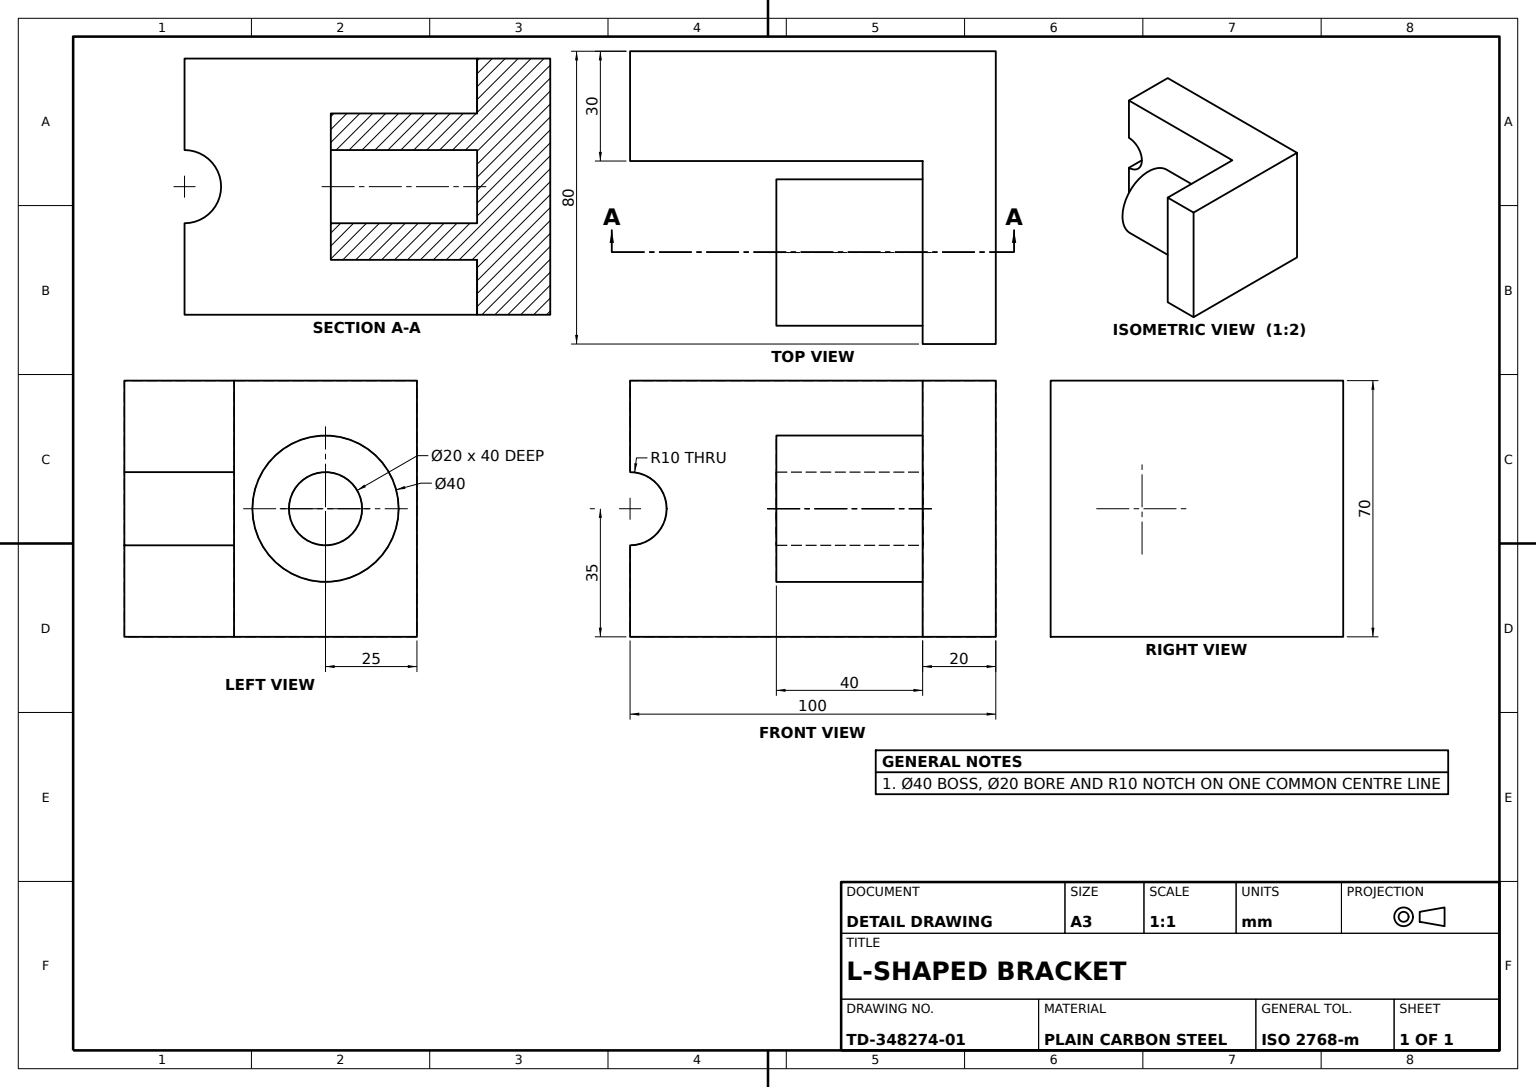
SolidWorks part; units mm, degrees
material "Plain Carbon Steel"
ref_plane "Front Plane" through (0, 0, 0) normal (0, 0, 1) x (1, 0, 0)
ref_plane "Top Plane" through (0, 0, 0) normal (0, 1, 0) x (1, 0, 0)
ref_plane "Right Plane" through (0, 0, 0) normal (1, 0, 0) x (0, 0, -1)
sketch "Base Plate Sketch" plane through (0, 0, 0) normal (0, 0, 1) x (1, 0, 0)
  line L0 (0, 0) -> (100, 0)
  line L1 (100, 0) -> (100, 70)
  line L2 (100, 70) -> (0, 70)
  line L3 (0, 70) -> (0, 0)
  dimension "D1" = 100
  dimension "D2" = 70
extrude "Base Plate" add sketch "Base Plate Sketch" along normal blind 30
sketch "Notch Sketch" plane through (0, 0, 30) normal (0, 0, 1) x (1, 0, 0)
  line L0 (0, 70) -> (0, 0) construction
  line L1 (0, 45) -> (0, 25)
  arc A0 (0, 25) -> (0, 45) centre (0, 35) ccw
  dimension "D1" = 20
  dimension "D2" = 10
extrude "Semicircular Notch" cut sketch "Notch Sketch" against normal blind 30
sketch "Upright Wall Sketch" plane through (100, 0, 0) normal (1, 0, 0) x (0, 0, -1)
  line L0 (-30, 70) -> (-80, 70)
  line L1 (-80, 70) -> (-80, 0)
  line L2 (-80, 0) -> (-30, 0)
  line L3 (-30, 0) -> (-30, 70) construction
  line L4 (-30, 0) -> (-30, 70)
  line L5 (0, 0) -> (0, 70) construction
  dimension "D1" = 80
extrude "Upright Wall" add sketch "Upright Wall Sketch" against normal blind 20
sketch "Half-Round Boss Sketch" plane through (80, 0, 0) normal (-1, 0, 0) x (0, 0, 1)
  line L0 (30, 0) -> (30, 70) construction
  line L1 (80, 0) -> (30, 0) construction
  circle A0 centre (55, 35) radius 20
  circle A1 centre (55, 35) radius 10
  dimension "D1" = 40
  dimension "D2" = 20
  dimension "D3" = 20
  dimension "D4" = 40
  dimension "D5" = 25
  dimension "D6" = 35
extrude "Half-Round Boss" add sketch "Half-Round Boss Sketch" along normal blind 40
